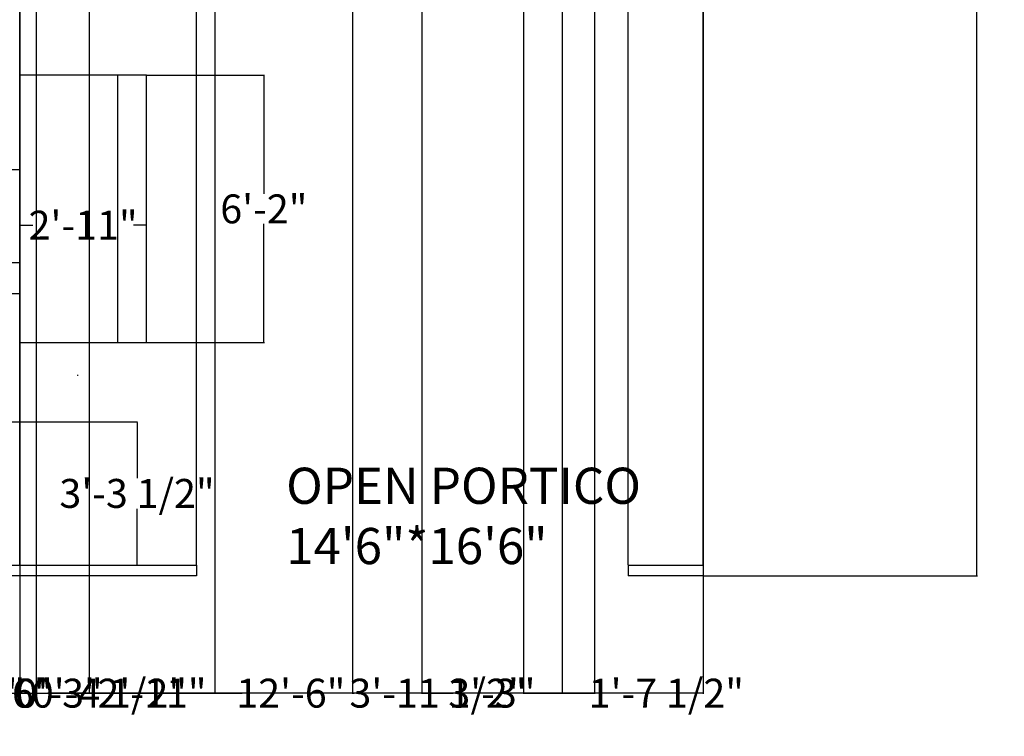
# Model space of a CAD drawing. Units: inches. Extents: x 3437 to 3994, y 3379 to 4084.
# Tile 3 of 6: x 3722 to 3994, y 3379 to 3577. Entities that reach past the tile are written whole.
import ezdxf

# ---------------------------------------------------------------- set-up
doc = ezdxf.new("R2010")
doc.units = ezdxf.units.IN
doc.header["$MEASUREMENT"] = 0
for name, color, linetype, lineweight in [('A-ANNO-DIMS', 2, 'Continuous', 18), ('A-AREA-IDEN', 7, 'Continuous', 25), ('A-FLOR-STRS', 7, 'Continuous', 25), ('C-PROP', 3, 'Continuous', 25)]:
    doc.layers.add(name, color=color, linetype=linetype, lineweight=lineweight)
doc.styles.get("Standard").update_dxf_attribs({"font": 'arial.ttf'})
doc.dimstyles.get("Standard").update_dxf_attribs({"dimtxt": 8, "dimasz": 0.18, "dimexe": 0.18, "dimexo": 0.0625, "dimgap": 0.09, "dimtad": 0, "dimtih": 1, "dimtoh": 1, "dimdec": 0, "dimzin": 0, "dimdsep": 46, "dimlunit": 3, "dimtxsty": 'Standard', "dimcen": 0.09, "dimadec": 0, "dimazin": 0, "dimtfac": 1, "dimtdec": 0, "dimtofl": 0, "dimtmove": 0, "dimatfit": 3, "dimfxl": 1, "dimtolj": 1, "dimtzin": 0, "dimarcsym": 0})

# ---------------------------------------------------------------- blocks, each defined once
blk = doc.blocks.new('*D10')
at = {"layer": 'A-ANNO-DIMS', "color": 0, "lineweight": -2, "transparency": 16777216}
for p, q in [((3911.09, 4023.64), (3986.96, 4023.64)), ((3986.78, 4023.46), (3986.78, 3727.81)), ((3986.78, 3423.82), (3986.78, 3719.46)), ((3911.09, 3423.64), (3986.96, 3423.64))]:
    blk.add_line(p, q, dxfattribs=at)
at = {"layer": 'A-ANNO-DIMS', "color": 0, "transparency": 16777216}
for points in [[(3986.75, 4023.46), (3986.81, 4023.46), (3986.78, 4023.64)], [(3986.75, 3423.82), (3986.81, 3423.82), (3986.78, 3423.64)]]:
    blk.add_solid(points, dxfattribs=at)
at = {"layer": 'Defpoints', "color": 0, "transparency": 16777216}
for p in [(3911.02, 4023.64), (3986.78, 4023.64), (3911.02, 3423.64)]:
    blk.add_point(p, dxfattribs=at)
at = {"layer": 'A-ANNO-DIMS', "color": 0, "transparency": 16777216, "insert": (3986.78, 3723.64), "char_height": 8, "attachment_point": 5}
blk.add_mtext("\\A1;50'", dxfattribs=at)
blk = doc.blocks.new('*D27')
at = {"layer": 'A-ANNO-DIMS', "color": 0, "lineweight": -2, "transparency": 16777216}
for p, q in [((3521.02, 3423.57), (3521.02, 3391.01)), ((3911.02, 3423.57), (3911.02, 3391.01)), ((3521.2, 3391.19), (3702.2, 3391.19)), ((3910.84, 3391.19), (3729.85, 3391.19))]:
    blk.add_line(p, q, dxfattribs=at)
at = {"layer": 'A-ANNO-DIMS', "color": 0, "transparency": 16777216}
for points in [[(3521.2, 3391.22), (3521.2, 3391.16), (3521.02, 3391.19)], [(3910.84, 3391.22), (3910.84, 3391.16), (3911.02, 3391.19)]]:
    blk.add_solid(points, dxfattribs=at)
at = {"layer": 'Defpoints', "color": 0, "transparency": 16777216}
for p in [(3521.02, 3423.64), (3911.02, 3423.64), (3911.02, 3391.19)]:
    blk.add_point(p, dxfattribs=at)
at = {"layer": 'A-ANNO-DIMS', "color": 0, "transparency": 16777216, "insert": (3716.02, 3391.19), "char_height": 8, "attachment_point": 5}
blk.add_mtext('\\A1;32\'-6"', dxfattribs=at)
blk = doc.blocks.new('*D46')
at = {"layer": 'A-ANNO-DIMS', "color": 0, "lineweight": -2, "transparency": 16777216}
for p, q in [((3576.02, 3426.7), (3576.02, 4056.27)), ((3576.2, 4056.09), (3635.57, 4056.09)), ((3721.84, 4056.09), (3662.48, 4056.09)), ((3722.02, 3426.7), (3722.02, 4056.27))]:
    blk.add_line(p, q, dxfattribs=at)
at = {"layer": 'A-ANNO-DIMS', "color": 0, "transparency": 16777216}
for points in [[(3576.2, 4056.12), (3576.2, 4056.06), (3576.02, 4056.09)], [(3721.84, 4056.12), (3721.84, 4056.06), (3722.02, 4056.09)]]:
    blk.add_solid(points, dxfattribs=at)
at = {"layer": 'Defpoints', "color": 0, "transparency": 16777216}
for p in [(3722.02, 4056.09), (3576.02, 3426.64), (3722.02, 3426.64)]:
    blk.add_point(p, dxfattribs=at)
at = {"layer": 'A-ANNO-DIMS', "color": 0, "transparency": 16777216, "insert": (3649.02, 4056.09), "char_height": 8, "attachment_point": 5}
blk.add_mtext('\\A1;12\'-2"', dxfattribs=at)
blk = doc.blocks.new('*D48')
at = {"layer": 'A-ANNO-DIMS', "color": 0, "lineweight": -2, "transparency": 16777216}
for p, q in [((3722.02, 3861.57), (3722.02, 3391.01)), ((3719.02, 3858.57), (3719.02, 3391.01)), ((3719.2, 3391.19), (3721.84, 3391.19)), ((3722.02, 3391.19), (3722.2, 3391.19))]:
    blk.add_line(p, q, dxfattribs=at)
at = {"layer": 'A-ANNO-DIMS', "color": 0, "transparency": 16777216}
for points in [[(3719.2, 3391.22), (3719.2, 3391.16), (3719.02, 3391.19)], [(3721.84, 3391.22), (3721.84, 3391.16), (3722.02, 3391.19)]]:
    blk.add_solid(points, dxfattribs=at)
at = {"layer": 'Defpoints', "color": 0, "transparency": 16777216}
for p in [(3722.02, 3861.64), (3719.02, 3858.64), (3722.02, 3391.19)]:
    blk.add_point(p, dxfattribs=at)
at = {"layer": 'A-ANNO-DIMS', "color": 0, "transparency": 16777216, "insert": (3732.93, 3391.19), "char_height": 8, "attachment_point": 5}
blk.add_mtext('\\A1;0\'-3"', dxfattribs=at)
blk = doc.blocks.new('*D51')
at = {"layer": 'A-ANNO-DIMS', "color": 0, "lineweight": -2, "transparency": 16777216}
for p, q in [((3814.05, 3618.57), (3814.05, 3391.01)), ((3861.41, 3618.57), (3861.41, 3391.01)), ((3814.23, 3391.19), (3814.58, 3391.19)), ((3861.23, 3391.19), (3860.88, 3391.19))]:
    blk.add_line(p, q, dxfattribs=at)
at = {"layer": 'A-ANNO-DIMS', "color": 0, "transparency": 16777216}
for points in [[(3814.23, 3391.22), (3814.23, 3391.16), (3814.05, 3391.19)], [(3861.23, 3391.22), (3861.23, 3391.16), (3861.41, 3391.19)]]:
    blk.add_solid(points, dxfattribs=at)
at = {"layer": 'Defpoints', "color": 0, "transparency": 16777216}
for p in [(3814.05, 3618.64), (3861.41, 3618.64), (3861.41, 3391.19)]:
    blk.add_point(p, dxfattribs=at)
at = {"layer": 'A-ANNO-DIMS', "color": 0, "transparency": 16777216, "insert": (3837.73, 3391.19), "char_height": 8, "attachment_point": 5}
blk.add_mtext('\\A1;3\'-11 1/2"', dxfattribs=at)
blk = doc.blocks.new('*D52')
at = {"layer": 'A-ANNO-DIMS', "color": 0, "lineweight": -2, "transparency": 16777216}
for p, q in [((3861.41, 3618.57), (3861.41, 3391.01)), ((3881.02, 3618.57), (3881.02, 3391.01)), ((3861.59, 3391.19), (3880.84, 3391.19)), ((3881.02, 3391.19), (3881.2, 3391.19))]:
    blk.add_line(p, q, dxfattribs=at)
at = {"layer": 'A-ANNO-DIMS', "color": 0, "transparency": 16777216}
for points in [[(3861.59, 3391.22), (3861.59, 3391.16), (3861.41, 3391.19)], [(3880.84, 3391.22), (3880.84, 3391.16), (3881.02, 3391.19)]]:
    blk.add_solid(points, dxfattribs=at)
at = {"layer": 'Defpoints', "color": 0, "transparency": 16777216}
for p in [(3861.41, 3618.64), (3881.02, 3618.64), (3881.02, 3391.19)]:
    blk.add_point(p, dxfattribs=at)
at = {"layer": 'A-ANNO-DIMS', "color": 0, "transparency": 16777216, "insert": (3900.87, 3391.19), "char_height": 8, "attachment_point": 5}
blk.add_mtext('\\A1;1\'-7 1/2"', dxfattribs=at)
blk = doc.blocks.new('*D53')
at = {"layer": 'A-ANNO-DIMS', "color": 0, "lineweight": -2, "transparency": 16777216}
for p, q in [((3770.9, 3426.7), (3770.9, 4056.27)), ((3771.08, 4056.09), (3807.48, 4056.09)), ((3890.18, 4056.09), (3853.78, 4056.09)), ((3890.36, 3426.7), (3890.36, 4056.27))]:
    blk.add_line(p, q, dxfattribs=at)
at = {"layer": 'A-ANNO-DIMS', "color": 0, "transparency": 16777216}
for points in [[(3771.08, 4056.12), (3771.08, 4056.06), (3770.9, 4056.09)], [(3890.18, 4056.12), (3890.18, 4056.06), (3890.36, 4056.09)]]:
    blk.add_solid(points, dxfattribs=at)
at = {"layer": 'Defpoints', "color": 0, "transparency": 16777216}
for p in [(3890.36, 4056.09), (3770.9, 3426.64), (3890.36, 3426.64)]:
    blk.add_point(p, dxfattribs=at)
at = {"layer": 'A-ANNO-DIMS', "color": 0, "transparency": 16777216, "insert": (3830.63, 4056.09), "char_height": 8, "attachment_point": 5}
blk.add_mtext('\\A1;9\'-11 1/2"', dxfattribs=at)
blk = doc.blocks.new('*D54')
at = {"layer": 'A-ANNO-DIMS', "color": 0, "lineweight": -2, "transparency": 16777216}
for p, q in [((3890.36, 3426.7), (3890.36, 4056.27)), ((3890.54, 4056.09), (3910.84, 4056.09)), ((3911.02, 3426.7), (3911.02, 4056.27)), ((3911.02, 4056.09), (3911.2, 4056.09))]:
    blk.add_line(p, q, dxfattribs=at)
at = {"layer": 'A-ANNO-DIMS', "color": 0, "transparency": 16777216}
for points in [[(3890.54, 4056.12), (3890.54, 4056.06), (3890.36, 4056.09)], [(3910.84, 4056.12), (3910.84, 4056.06), (3911.02, 4056.09)]]:
    blk.add_solid(points, dxfattribs=at)
at = {"layer": 'Defpoints', "color": 0, "transparency": 16777216}
for p in [(3911.02, 4056.09), (3890.36, 3426.64), (3911.02, 3426.64)]:
    blk.add_point(p, dxfattribs=at)
at = {"layer": 'A-ANNO-DIMS', "color": 0, "transparency": 16777216, "insert": (3930.87, 4056.09), "char_height": 8, "attachment_point": 5}
blk.add_mtext('\\A1;1\'-8 1/2"', dxfattribs=at)
blk = doc.blocks.new('*D57')
at = {"layer": 'A-ANNO-DIMS', "color": 0, "lineweight": -2, "transparency": 16777216}
for p, q in [((3741.22, 3861.57), (3741.22, 3391.01)), ((3776.02, 3861.57), (3776.02, 3391.01)), ((3741.4, 3391.19), (3744.72, 3391.19)), ((3775.84, 3391.19), (3772.52, 3391.19))]:
    blk.add_line(p, q, dxfattribs=at)
at = {"layer": 'A-ANNO-DIMS', "color": 0, "transparency": 16777216}
for points in [[(3741.4, 3391.22), (3741.4, 3391.16), (3741.22, 3391.19)], [(3775.84, 3391.22), (3775.84, 3391.16), (3776.02, 3391.19)]]:
    blk.add_solid(points, dxfattribs=at)
at = {"layer": 'Defpoints', "color": 0, "transparency": 16777216}
for p in [(3741.22, 3861.64), (3776.02, 3861.64), (3776.02, 3391.19)]:
    blk.add_point(p, dxfattribs=at)
at = {"layer": 'A-ANNO-DIMS', "color": 0, "transparency": 16777216, "insert": (3758.62, 3391.19), "char_height": 8, "attachment_point": 5}
blk.add_mtext('\\A1;2\'-11"', dxfattribs=at)
blk = doc.blocks.new('*D62')
at = {"layer": 'A-ANNO-DIMS', "color": 0, "lineweight": -2, "transparency": 16777216}
for p, q in [((3721.96, 3535.98), (3689.39, 3535.98)), ((3689.57, 3535.8), (3689.57, 3527.35)), ((3689.57, 3510.44), (3689.57, 3518.9)), ((3721.96, 3510.26), (3689.39, 3510.26))]:
    blk.add_line(p, q, dxfattribs=at)
at = {"layer": 'A-ANNO-DIMS', "color": 0, "transparency": 16777216}
for points in [[(3689.54, 3535.8), (3689.6, 3535.8), (3689.57, 3535.98)], [(3689.54, 3510.44), (3689.6, 3510.44), (3689.57, 3510.26)]]:
    blk.add_solid(points, dxfattribs=at)
at = {"layer": 'Defpoints', "color": 0, "transparency": 16777216}
for p in [(3689.57, 3535.98), (3722.02, 3535.98), (3722.02, 3510.26)]:
    blk.add_point(p, dxfattribs=at)
at = {"layer": 'A-ANNO-DIMS', "color": 0, "transparency": 16777216, "insert": (3689.57, 3523.12), "char_height": 8, "attachment_point": 5}
blk.add_mtext('\\A1;2\'-1 1/2"', dxfattribs=at)
blk = doc.blocks.new('*D67')
at = {"layer": 'A-ANNO-DIMS', "color": 0, "lineweight": -2, "transparency": 16777216}
for p, q in [((3722.02, 3488.26), (3722.02, 3520.83)), ((3722.2, 3520.65), (3725.67, 3520.65)), ((3756.93, 3520.65), (3753.46, 3520.65)), ((3757.11, 3488.26), (3757.11, 3520.83))]:
    blk.add_line(p, q, dxfattribs=at)
at = {"layer": 'A-ANNO-DIMS', "color": 0, "transparency": 16777216}
for points in [[(3722.2, 3520.68), (3722.2, 3520.62), (3722.02, 3520.65)], [(3756.93, 3520.68), (3756.93, 3520.62), (3757.11, 3520.65)]]:
    blk.add_solid(points, dxfattribs=at)
at = {"layer": 'Defpoints', "color": 0, "transparency": 16777216}
for p in [(3757.11, 3520.65), (3722.02, 3488.2), (3757.11, 3488.2)]:
    blk.add_point(p, dxfattribs=at)
at = {"layer": 'A-ANNO-DIMS', "color": 0, "transparency": 16777216, "insert": (3739.57, 3520.65), "char_height": 8, "attachment_point": 5}
blk.add_mtext('\\A1;2\'-11"', dxfattribs=at)
blk = doc.blocks.new('*D68')
at = {"layer": 'A-ANNO-DIMS', "color": 0, "lineweight": -2, "transparency": 16777216}
for p, q in [((3757.17, 3562.1), (3789.74, 3562.1)), ((3789.56, 3561.92), (3789.56, 3529.32)), ((3789.56, 3488.38), (3789.56, 3520.98)), ((3757.17, 3488.2), (3789.74, 3488.2))]:
    blk.add_line(p, q, dxfattribs=at)
at = {"layer": 'A-ANNO-DIMS', "color": 0, "transparency": 16777216}
for points in [[(3789.53, 3561.92), (3789.59, 3561.92), (3789.56, 3562.1)], [(3789.53, 3488.38), (3789.59, 3488.38), (3789.56, 3488.2)]]:
    blk.add_solid(points, dxfattribs=at)
at = {"layer": 'Defpoints', "color": 0, "transparency": 16777216}
for p in [(3757.11, 3562.1), (3757.11, 3488.2), (3789.56, 3488.2)]:
    blk.add_point(p, dxfattribs=at)
at = {"layer": 'A-ANNO-DIMS', "color": 0, "transparency": 16777216, "insert": (3789.56, 3525.15), "char_height": 8, "attachment_point": 5}
blk.add_mtext('\\A1;6\'-2"', dxfattribs=at)
blk = doc.blocks.new('*D70')
at = {"layer": 'A-ANNO-DIMS', "color": 0, "lineweight": -2, "transparency": 16777216}
for p, q in [((3722.09, 3466.24), (3754.65, 3466.24)), ((3754.47, 3466.06), (3754.47, 3450.67)), ((3754.47, 3426.82), (3754.47, 3442.21)), ((3722.09, 3426.64), (3754.65, 3426.64))]:
    blk.add_line(p, q, dxfattribs=at)
at = {"layer": 'A-ANNO-DIMS', "color": 0, "transparency": 16777216}
for points in [[(3754.44, 3466.06), (3754.5, 3466.06), (3754.47, 3466.24)], [(3754.44, 3426.82), (3754.5, 3426.82), (3754.47, 3426.64)]]:
    blk.add_solid(points, dxfattribs=at)
at = {"layer": 'Defpoints', "color": 0, "transparency": 16777216}
for p in [(3722.02, 3466.24), (3722.02, 3426.64), (3754.47, 3426.64)]:
    blk.add_point(p, dxfattribs=at)
at = {"layer": 'A-ANNO-DIMS', "color": 0, "transparency": 16777216, "insert": (3754.47, 3446.44), "char_height": 8, "attachment_point": 5}
blk.add_mtext('\\A1;3\'-3 1/2"', dxfattribs=at)
blk = doc.blocks.new('*D76')
at = {"layer": 'A-ANNO-DIMS', "color": 0, "lineweight": -2, "transparency": 16777216}
for p, q in [((3689.57, 3510.44), (3689.57, 3510.62)), ((3721.96, 3510.26), (3689.39, 3510.26)), ((3721.96, 3501.64), (3689.39, 3501.64)), ((3689.57, 3501.46), (3689.57, 3501.28))]:
    blk.add_line(p, q, dxfattribs=at)
at = {"layer": 'A-ANNO-DIMS', "color": 0, "transparency": 16777216}
for points in [[(3689.54, 3510.44), (3689.6, 3510.44), (3689.57, 3510.26)], [(3689.54, 3501.46), (3689.6, 3501.46), (3689.57, 3501.64)]]:
    blk.add_solid(points, dxfattribs=at)
at = {"layer": 'Defpoints', "color": 0, "transparency": 16777216}
for p in [(3689.57, 3510.26), (3722.02, 3510.26), (3722.02, 3501.64)]:
    blk.add_point(p, dxfattribs=at)
at = {"layer": 'A-ANNO-DIMS', "color": 0, "transparency": 16777216, "insert": (3689.57, 3505.95), "char_height": 8, "attachment_point": 5}
blk.add_mtext('\\A1;0\'-8 1/2"', dxfattribs=at)
blk = doc.blocks.new('*D79')
at = {"layer": 'A-ANNO-DIMS', "color": 0, "lineweight": -2, "transparency": 16777216}
for p, q in [((3675.76, 3905.25), (3675.76, 3391.01)), ((3665.02, 3903.57), (3665.02, 3391.01)), ((3665.2, 3391.19), (3675.58, 3391.19)), ((3675.76, 3391.19), (3675.94, 3391.19))]:
    blk.add_line(p, q, dxfattribs=at)
at = {"layer": 'A-ANNO-DIMS', "color": 0, "transparency": 16777216}
for points in [[(3665.2, 3391.22), (3665.2, 3391.16), (3665.02, 3391.19)], [(3675.58, 3391.22), (3675.58, 3391.16), (3675.76, 3391.19)]]:
    blk.add_solid(points, dxfattribs=at)
at = {"layer": 'Defpoints', "color": 0, "transparency": 16777216}
for p in [(3675.76, 3905.31), (3665.02, 3903.64), (3675.76, 3391.19)]:
    blk.add_point(p, dxfattribs=at)
at = {"layer": 'A-ANNO-DIMS', "color": 0, "transparency": 16777216, "insert": (3699.09, 3391.19), "char_height": 8, "attachment_point": 5}
blk.add_mtext('\\A1;0\'-10 1/2"', dxfattribs=at)
blk = doc.blocks.new('*D81')
at = {"layer": 'A-ANNO-DIMS', "color": 0, "lineweight": -2, "transparency": 16777216}
for p, q in [((3722.02, 3984.57), (3722.02, 3391.01)), ((3872.02, 3984.57), (3872.02, 3391.01)), ((3722.2, 3391.19), (3783.57, 3391.19)), ((3871.84, 3391.19), (3810.48, 3391.19))]:
    blk.add_line(p, q, dxfattribs=at)
at = {"layer": 'A-ANNO-DIMS', "color": 0, "transparency": 16777216}
for points in [[(3722.2, 3391.22), (3722.2, 3391.16), (3722.02, 3391.19)], [(3871.84, 3391.22), (3871.84, 3391.16), (3872.02, 3391.19)]]:
    blk.add_solid(points, dxfattribs=at)
at = {"layer": 'Defpoints', "color": 0, "transparency": 16777216}
for p in [(3722.02, 3984.64), (3872.02, 3984.64), (3872.02, 3391.19)]:
    blk.add_point(p, dxfattribs=at)
at = {"layer": 'A-ANNO-DIMS', "color": 0, "transparency": 16777216, "insert": (3797.02, 3391.19), "char_height": 8, "attachment_point": 5}
blk.add_mtext('\\A1;12\'-6"', dxfattribs=at)
blk = doc.blocks.new('*D84')
at = {"layer": 'A-ANNO-DIMS', "color": 0, "lineweight": -2, "transparency": 16777216}
for p, q in [((3726.61, 3637.53), (3726.61, 3391.01)), ((3722.02, 3621.57), (3722.02, 3391.01)), ((3722.2, 3391.19), (3726.43, 3391.19)), ((3726.61, 3391.19), (3726.79, 3391.19))]:
    blk.add_line(p, q, dxfattribs=at)
at = {"layer": 'A-ANNO-DIMS', "color": 0, "transparency": 16777216}
for points in [[(3722.2, 3391.22), (3722.2, 3391.16), (3722.02, 3391.19)], [(3726.43, 3391.22), (3726.43, 3391.16), (3726.61, 3391.19)]]:
    blk.add_solid(points, dxfattribs=at)
at = {"layer": 'Defpoints', "color": 0, "transparency": 16777216}
for p in [(3726.61, 3637.59), (3722.02, 3621.64), (3726.61, 3391.19)]:
    blk.add_point(p, dxfattribs=at)
at = {"layer": 'A-ANNO-DIMS', "color": 0, "transparency": 16777216, "insert": (3746.84, 3391.19), "char_height": 8, "attachment_point": 5}
blk.add_mtext('\\A1;0\'-4 1/2"', dxfattribs=at)
blk = doc.blocks.new('*D85')
at = {"layer": 'A-ANNO-DIMS', "color": 0, "lineweight": -2, "transparency": 16777216}
for p, q in [((3872.02, 3730.32), (3872.02, 3391.01)), ((3833.23, 3722.95), (3833.23, 3391.01)), ((3833.41, 3391.19), (3841.91, 3391.19)), ((3871.84, 3391.19), (3863.35, 3391.19))]:
    blk.add_line(p, q, dxfattribs=at)
at = {"layer": 'A-ANNO-DIMS', "color": 0, "transparency": 16777216}
for points in [[(3833.41, 3391.22), (3833.41, 3391.16), (3833.23, 3391.19)], [(3871.84, 3391.22), (3871.84, 3391.16), (3872.02, 3391.19)]]:
    blk.add_solid(points, dxfattribs=at)
at = {"layer": 'Defpoints', "color": 0, "transparency": 16777216}
for p in [(3872.02, 3730.38), (3833.23, 3723.01), (3872.02, 3391.19)]:
    blk.add_point(p, dxfattribs=at)
at = {"layer": 'A-ANNO-DIMS', "color": 0, "transparency": 16777216, "insert": (3852.63, 3391.19), "char_height": 8, "attachment_point": 5}
blk.add_mtext('\\A1;3\'-3"', dxfattribs=at)
blk = doc.blocks.new('*D88')
at = {"layer": 'A-ANNO-DIMS', "color": 0, "lineweight": -2, "transparency": 16777216}
for p, q in [((3681.05, 3554.61), (3681.23, 3554.61)), ((3681.23, 3554.61), (3702.45, 3526.46)), ((3738.02, 3479.16), (3738.2, 3479.16)), ((3738.11, 3479.07), (3738.11, 3479.25))]:
    blk.add_line(p, q, dxfattribs=at)
at = {"layer": 'A-ANNO-DIMS', "color": 0, "transparency": 16777216}
blk.add_solid([(3702.48, 3526.48), (3702.43, 3526.44), (3702.56, 3526.32)], dxfattribs=at)
at = {"layer": 'Defpoints', "color": 0, "transparency": 16777216}
for p in [(3702.56, 3526.32), (3738.11, 3479.16)]:
    blk.add_point(p, dxfattribs=at)
at = {"layer": 'A-ANNO-DIMS', "color": 0, "transparency": 16777216, "insert": (3663.39, 3554.61), "char_height": 8, "attachment_point": 5}
blk.add_mtext('\\A1;R4\'-11"', dxfattribs=at)

msp = doc.modelspace()

# ---------------------------------------------------------------- linework, layer by layer
at = {"layer": 'A-FLOR-STRS'}
for p, q in [((3757.11, 3562.1), (3722.02, 3562.1)), ((3749.07, 3562.1), (3749.07, 3488.2)), ((3757.11, 3488.2), (3757.11, 3562.1)), ((3722.02, 3535.98), (3722.02, 3488.2)), ((3722.02, 3488.2), (3757.11, 3488.2)), ((3722.02, 3488.2), (3722.02, 3426.64)), ((3576.02, 3466.24), (3722.02, 3466.24))]:
    msp.add_line(p, q, dxfattribs=at)
at = {"layer": 'C-PROP'}
for p, q in [((3911.02, 4023.64), (3911.02, 3426.64)), ((3530.02, 3426.64), (3770.9, 3426.64)), ((3770.9, 3426.64), (3770.9, 3423.64)), ((3890.36, 3426.64), (3899.69, 3426.64)), ((3890.36, 3426.64), (3890.36, 3423.64)), ((3899.69, 3426.64), (3911.02, 3426.64))]:
    msp.add_line(p, q, dxfattribs=at)
msp.add_lwpolyline([(3770.9, 3423.64), (3491.02, 3423.64), (3491.02, 4023.64), (3911.02, 4023.64), (3911.02, 3423.64), (3890.36, 3423.64)], dxfattribs=at)

# ---------------------------------------------------------------- texts
at = {"layer": 'A-AREA-IDEN', "insert": (3795.73, 3453.56), "char_height": 10, "attachment_point": 1}
msp.add_mtext_dynamic_manual_height_columns('OPEN PORTICO\\P14\'6"*16\'6"', width=200.853, gutter_width=1, heights=[0], dxfattribs=at)

# ---------------------------------------------------------------- dimensions: what is measured, and where the dimension line sits
at = {"layer": 'A-ANNO-DIMS'}
for base, p1, p2, picture, middle in [((3890.36, 4056.09), (3770.9, 3426.64), (3890.36, 3426.64), '*D53', (3830.63, 4056.09)), ((3911.02, 4056.09), (3890.36, 3426.64), (3911.02, 3426.64), '*D54', (3930.87, 4056.09)), ((3722.02, 4056.09), (3576.02, 3426.64), (3722.02, 3426.64), '*D46', (3649.02, 4056.09)), ((3872.02, 3391.19), (3722.02, 3984.64), (3872.02, 3984.64), '*D81', (3797.02, 3391.19)), ((3675.76, 3391.19), (3665.02, 3903.64), (3675.76, 3905.31), '*D79', (3699.09, 3391.19)), ((3722.02, 3391.19), (3719.02, 3858.64), (3722.02, 3861.64), '*D48', (3732.93, 3391.19)), ((3776.02, 3391.19), (3741.22, 3861.64), (3776.02, 3861.64), '*D57', (3758.62, 3391.19)), ((3872.02, 3391.19), (3833.23, 3723.01), (3872.02, 3730.38), '*D85', (3852.63, 3391.19)), ((3726.61, 3391.19), (3722.02, 3621.64), (3726.61, 3637.59), '*D84', (3746.84, 3391.19)), ((3861.41, 3391.19), (3814.05, 3618.64), (3861.41, 3618.64), '*D51', (3837.73, 3391.19)), ((3881.02, 3391.19), (3861.41, 3618.64), (3881.02, 3618.64), '*D52', (3900.87, 3391.19)), ((3757.11, 3520.65), (3722.02, 3488.2), (3757.11, 3488.2), '*D67', (3739.57, 3520.65)), ((3911.02, 3391.19), (3521.02, 3423.64), (3911.02, 3423.64), '*D27', (3716.02, 3391.19))]:
    dim = msp.add_linear_dim(base=base, p1=p1, p2=p2, dimstyle='Standard', override={"dimdec": 1, "dimlfac": 1, "dimrnd": 0, "dimzin": 1, "dimdsep": 46, "dimlunit": 4, "dimfrac": 2}, dxfattribs=at)
    dim.commit()
    dim.dimension.update_dxf_attribs({"geometry": picture, "text_midpoint": middle})
for base, p1, p2, angle, override, picture, middle in [((3986.78, 4023.64), (3911.02, 3423.64), (3911.02, 4023.64), 90, {"dimclrd": 0, "dimclre": 0, "dimclrt": 0}, '*D10', (3986.78, 3723.64)), ((3789.56, 3488.2), (3757.11, 3562.1), (3757.11, 3488.2), 270, {"dimdec": 1, "dimlfac": 1, "dimrnd": 0, "dimzin": 1, "dimdsep": 46, "dimlunit": 4, "dimfrac": 2}, '*D68', (3789.56, 3525.15)), ((3689.57, 3535.98), (3722.02, 3510.26), (3722.02, 3535.98), 90, {"dimdec": 1, "dimlfac": 1, "dimrnd": 0, "dimzin": 1, "dimdsep": 46, "dimlunit": 4, "dimfrac": 2}, '*D62', (3689.57, 3523.12)), ((3689.57, 3510.26), (3722.02, 3501.64), (3722.02, 3510.26), 90, {"dimdec": 1, "dimlfac": 1, "dimrnd": 0, "dimzin": 1, "dimdsep": 46, "dimlunit": 4, "dimfrac": 2}, '*D76', (3689.57, 3505.95)), ((3754.47, 3426.64), (3722.02, 3466.24), (3722.02, 3426.64), 270, {"dimdec": 1, "dimlfac": 1, "dimrnd": 0, "dimzin": 1, "dimdsep": 46, "dimlunit": 4, "dimfrac": 2}, '*D70', (3754.47, 3446.44))]:
    dim = msp.add_linear_dim(base=base, p1=p1, p2=p2, angle=angle, dimstyle='Standard', override=override, dxfattribs=at)
    dim.commit()
    dim.dimension.update_dxf_attribs({"geometry": picture, "text_midpoint": middle})
dim = msp.add_radius_dim(center=(3738.11, 3479.16), mpoint=(3702.56, 3526.32), dimstyle='Standard', override={"dimdec": 1, "dimlfac": 1, "dimrnd": 0, "dimzin": 1, "dimdsep": 46, "dimlunit": 4, "dimfrac": 2}, dxfattribs=at)
dim.commit()
dim.dimension.update_dxf_attribs({"geometry": '*D88', "text_midpoint": (3663.39, 3554.61), "dimtype": 164})

doc.saveas('drawing.dxf')
